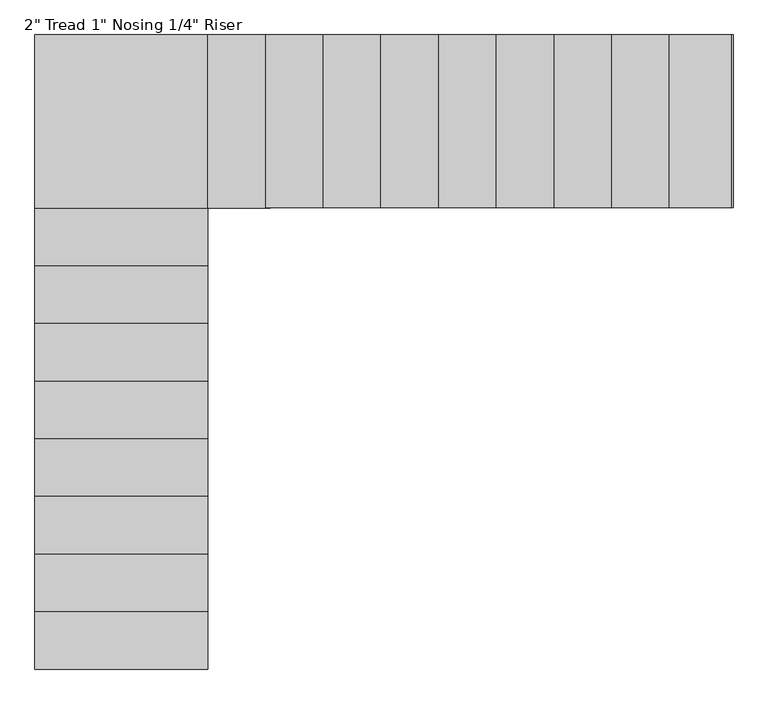
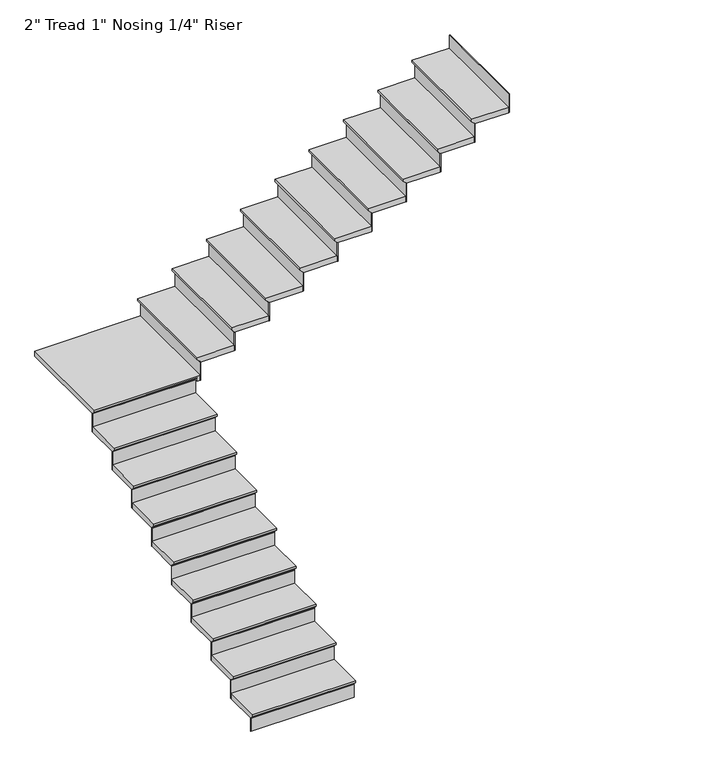
"""IFC4 building model written with IfcOpenShell, lengths in millimetres: stair flight geometry."""

from ifc_helpers import new_model, si_unit, origin, place, context, project, spatial, faceted_brep, source, transform, mapped, element, save


def stair_flight_ebba5fc4(model_context):
    return source(origin(), model_context, "Body", "Brep", [
        faceted_brep([(-6027.2757327, 1771.427543, 3506.47), (-6027.2757327, 1771.427543, 3525.52), (-6941.6757327, 1771.427543, 3525.52), (-6941.6757327, 1771.427543, 3506.47), (-6027.2757327, 1796.827543, 3481.07), (-6941.6757327, 1796.827543, 3481.07), (-6027.2757327, 2101.627543, 3525.52), (-6941.6757327, 2101.627543, 3525.52), (-6941.6757327, 1796.827543, 3474.72), (-6941.6757327, 2101.627543, 3474.72), (-6027.2757327, 2101.627543, 3474.72), (-6027.2757327, 1796.827543, 3474.72)], [[[0, 1, 2, 3]], [[4, 0, 3, 5]], [[2, 1, 6, 7]], [[8, 9, 10, 11]], [[2, 7, 9, 8, 5, 3]], [[8, 11, 4, 5]], [[6, 1, 0, 4, 11, 10]], [[7, 6, 10, 9]]]),
        faceted_brep([(-6027.2757327, 1796.827543, 3474.72), (-6027.2757327, 1796.827543, 3352.8), (-6027.2757327, 1803.177543, 3352.8), (-6027.2757327, 1803.177543, 3474.72), (-6941.6757327, 1796.827543, 3474.72), (-6941.6757327, 1803.177543, 3474.72), (-6941.6757327, 1803.177543, 3352.8), (-6941.6757327, 1796.827543, 3352.8)], [[[0, 1, 2, 3]], [[4, 5, 6, 7]], [[1, 0, 4, 7]], [[2, 1, 7, 6]], [[3, 2, 6, 5]], [[0, 3, 5, 4]]]),
        faceted_brep([(-6027.2757327, 2101.627543, 3647.44), (-6027.2757327, 2101.627543, 3474.72), (-6027.2757327, 2107.977543, 3474.72), (-6027.2757327, 2107.977543, 3647.44), (-6941.6757327, 2101.627543, 3647.44), (-6941.6757327, 2107.977543, 3647.44), (-6941.6757327, 2107.977543, 3474.72), (-6941.6757327, 2101.627543, 3474.72)], [[[0, 1, 2, 3]], [[4, 5, 6, 7]], [[1, 0, 4, 7]], [[2, 1, 7, 6]], [[3, 2, 6, 5]], [[0, 3, 5, 4]]]),
        faceted_brep([(-6941.6757327, 2076.227543, 3698.24), (-6027.2757327, 2076.227543, 3698.24), (-6027.2757327, 2406.427543, 3698.24), (-6941.6757327, 2406.427543, 3698.24), (-6941.6757327, 2101.627543, 3647.44), (-6941.6757327, 2406.427543, 3647.44), (-6027.2757327, 2406.427543, 3647.44), (-6027.2757327, 2101.627543, 3647.44), (-6941.6757327, 2101.627543, 3653.79), (-6941.6757327, 2076.227543, 3679.19), (-6027.2757327, 2101.627543, 3653.79), (-6027.2757327, 2076.227543, 3679.19)], [[[0, 1, 2, 3]], [[4, 5, 6, 7]], [[0, 3, 5, 4, 8, 9]], [[4, 7, 10, 8]], [[2, 1, 11, 10, 7, 6]], [[3, 2, 6, 5]], [[11, 1, 0, 9]], [[10, 11, 9, 8]]]),
        faceted_brep([(-6027.2757327, 2406.427543, 3820.16), (-6027.2757327, 2406.427543, 3647.44), (-6027.2757327, 2412.777543, 3647.44), (-6027.2757327, 2412.777543, 3820.16), (-6941.6757327, 2406.427543, 3820.16), (-6941.6757327, 2412.777543, 3820.16), (-6941.6757327, 2412.777543, 3647.44), (-6941.6757327, 2406.427543, 3647.44)], [[[0, 1, 2, 3]], [[4, 5, 6, 7]], [[1, 0, 4, 7]], [[2, 1, 7, 6]], [[3, 2, 6, 5]], [[0, 3, 5, 4]]]),
        faceted_brep([(-6941.6757327, 2381.027543, 3870.96), (-6027.2757327, 2381.027543, 3870.96), (-6027.2757327, 2711.227543, 3870.96), (-6941.6757327, 2711.227543, 3870.96), (-6941.6757327, 2406.427543, 3820.16), (-6941.6757327, 2711.227543, 3820.16), (-6027.2757327, 2711.227543, 3820.16), (-6027.2757327, 2406.427543, 3820.16), (-6941.6757327, 2406.427543, 3826.51), (-6941.6757327, 2381.027543, 3851.91), (-6027.2757327, 2406.427543, 3826.51), (-6027.2757327, 2381.027543, 3851.91)], [[[0, 1, 2, 3]], [[4, 5, 6, 7]], [[0, 3, 5, 4, 8, 9]], [[4, 7, 10, 8]], [[2, 1, 11, 10, 7, 6]], [[3, 2, 6, 5]], [[11, 1, 0, 9]], [[10, 11, 9, 8]]]),
        faceted_brep([(-6027.2757327, 2711.227543, 3992.88), (-6027.2757327, 2711.227543, 3820.16), (-6027.2757327, 2717.577543, 3820.16), (-6027.2757327, 2717.577543, 3992.88), (-6941.6757327, 2711.227543, 3992.88), (-6941.6757327, 2717.577543, 3992.88), (-6941.6757327, 2717.577543, 3820.16), (-6941.6757327, 2711.227543, 3820.16)], [[[0, 1, 2, 3]], [[4, 5, 6, 7]], [[1, 0, 4, 7]], [[2, 1, 7, 6]], [[3, 2, 6, 5]], [[0, 3, 5, 4]]]),
        faceted_brep([(-6941.6757327, 2685.827543, 4043.68), (-6027.2757327, 2685.827543, 4043.68), (-6027.2757327, 3016.027543, 4043.68), (-6941.6757327, 3016.027543, 4043.68), (-6941.6757327, 2711.227543, 3992.88), (-6941.6757327, 3016.027543, 3992.88), (-6027.2757327, 3016.027543, 3992.88), (-6027.2757327, 2711.227543, 3992.88), (-6941.6757327, 2711.227543, 3999.23), (-6941.6757327, 2685.827543, 4024.63), (-6027.2757327, 2711.227543, 3999.23), (-6027.2757327, 2685.827543, 4024.63)], [[[0, 1, 2, 3]], [[4, 5, 6, 7]], [[0, 3, 5, 4, 8, 9]], [[4, 7, 10, 8]], [[2, 1, 11, 10, 7, 6]], [[3, 2, 6, 5]], [[11, 1, 0, 9]], [[10, 11, 9, 8]]]),
        faceted_brep([(-6027.2757327, 3016.027543, 4165.6), (-6027.2757327, 3016.027543, 3992.88), (-6027.2757327, 3022.377543, 3992.88), (-6027.2757327, 3022.377543, 4165.6), (-6941.6757327, 3016.027543, 4165.6), (-6941.6757327, 3022.377543, 4165.6), (-6941.6757327, 3022.377543, 3992.88), (-6941.6757327, 3016.027543, 3992.88)], [[[0, 1, 2, 3]], [[4, 5, 6, 7]], [[1, 0, 4, 7]], [[2, 1, 7, 6]], [[3, 2, 6, 5]], [[0, 3, 5, 4]]]),
        faceted_brep([(-6941.6757327, 2990.627543, 4216.4), (-6027.2757327, 2990.627543, 4216.4), (-6027.2757327, 3320.827543, 4216.4), (-6941.6757327, 3320.827543, 4216.4), (-6941.6757327, 3016.027543, 4165.6), (-6941.6757327, 3320.827543, 4165.6), (-6027.2757327, 3320.827543, 4165.6), (-6027.2757327, 3016.027543, 4165.6), (-6941.6757327, 3016.027543, 4171.95), (-6941.6757327, 2990.627543, 4197.35), (-6027.2757327, 3016.027543, 4171.95), (-6027.2757327, 2990.627543, 4197.35)], [[[0, 1, 2, 3]], [[4, 5, 6, 7]], [[0, 3, 5, 4, 8, 9]], [[4, 7, 10, 8]], [[2, 1, 11, 10, 7, 6]], [[3, 2, 6, 5]], [[11, 1, 0, 9]], [[10, 11, 9, 8]]]),
        faceted_brep([(-6027.2757327, 3320.827543, 4338.32), (-6027.2757327, 3320.827543, 4165.6), (-6027.2757327, 3327.177543, 4165.6), (-6027.2757327, 3327.177543, 4338.32), (-6941.6757327, 3320.827543, 4338.32), (-6941.6757327, 3327.177543, 4338.32), (-6941.6757327, 3327.177543, 4165.6), (-6941.6757327, 3320.827543, 4165.6)], [[[0, 1, 2, 3]], [[4, 5, 6, 7]], [[1, 0, 4, 7]], [[2, 1, 7, 6]], [[3, 2, 6, 5]], [[0, 3, 5, 4]]]),
        faceted_brep([(-6941.6757327, 3295.427543, 4389.12), (-6027.2757327, 3295.427543, 4389.12), (-6027.2757327, 3625.627543, 4389.12), (-6941.6757327, 3625.627543, 4389.12), (-6941.6757327, 3320.827543, 4338.32), (-6941.6757327, 3625.627543, 4338.32), (-6027.2757327, 3625.627543, 4338.32), (-6027.2757327, 3320.827543, 4338.32), (-6941.6757327, 3320.827543, 4344.67), (-6941.6757327, 3295.427543, 4370.07), (-6027.2757327, 3320.827543, 4344.67), (-6027.2757327, 3295.427543, 4370.07)], [[[0, 1, 2, 3]], [[4, 5, 6, 7]], [[0, 3, 5, 4, 8, 9]], [[4, 7, 10, 8]], [[2, 1, 11, 10, 7, 6]], [[3, 2, 6, 5]], [[11, 1, 0, 9]], [[10, 11, 9, 8]]]),
        faceted_brep([(-6027.2757327, 3625.627543, 4511.04), (-6027.2757327, 3625.627543, 4338.32), (-6027.2757327, 3631.977543, 4338.32), (-6027.2757327, 3631.977543, 4511.04), (-6941.6757327, 3625.627543, 4511.04), (-6941.6757327, 3631.977543, 4511.04), (-6941.6757327, 3631.977543, 4338.32), (-6941.6757327, 3625.627543, 4338.32)], [[[0, 1, 2, 3]], [[4, 5, 6, 7]], [[1, 0, 4, 7]], [[2, 1, 7, 6]], [[3, 2, 6, 5]], [[0, 3, 5, 4]]]),
        faceted_brep([(-6941.6757327, 3600.227543, 4561.84), (-6027.2757327, 3600.227543, 4561.84), (-6027.2757327, 3930.427543, 4561.84), (-6941.6757327, 3930.427543, 4561.84), (-6941.6757327, 3625.627543, 4511.04), (-6941.6757327, 3930.427543, 4511.04), (-6027.2757327, 3930.427543, 4511.04), (-6027.2757327, 3625.627543, 4511.04), (-6941.6757327, 3625.627543, 4517.39), (-6941.6757327, 3600.227543, 4542.79), (-6027.2757327, 3625.627543, 4517.39), (-6027.2757327, 3600.227543, 4542.79)], [[[0, 1, 2, 3]], [[4, 5, 6, 7]], [[0, 3, 5, 4, 8, 9]], [[4, 7, 10, 8]], [[2, 1, 11, 10, 7, 6]], [[3, 2, 6, 5]], [[11, 1, 0, 9]], [[10, 11, 9, 8]]]),
        faceted_brep([(-6027.2757327, 3930.427543, 4683.76), (-6027.2757327, 3930.427543, 4511.04), (-6027.2757327, 3936.777543, 4511.04), (-6027.2757327, 3936.777543, 4683.76), (-6941.6757327, 3930.427543, 4683.76), (-6941.6757327, 3936.777543, 4683.76), (-6941.6757327, 3936.777543, 4511.04), (-6941.6757327, 3930.427543, 4511.04)], [[[0, 1, 2, 3]], [[4, 5, 6, 7]], [[1, 0, 4, 7]], [[2, 1, 7, 6]], [[3, 2, 6, 5]], [[0, 3, 5, 4]]]),
        faceted_brep([(-6941.6757327, 3905.027543, 4734.56), (-6027.2757327, 3905.027543, 4734.56), (-6027.2757327, 4235.227543, 4734.56), (-6941.6757327, 4235.227543, 4734.56), (-6941.6757327, 3930.427543, 4683.76), (-6941.6757327, 4235.227543, 4683.76), (-6027.2757327, 4235.227543, 4683.76), (-6027.2757327, 3930.427543, 4683.76), (-6941.6757327, 3930.427543, 4690.11), (-6941.6757327, 3905.027543, 4715.51), (-6027.2757327, 3930.427543, 4690.11), (-6027.2757327, 3905.027543, 4715.51)], [[[0, 1, 2, 3]], [[4, 5, 6, 7]], [[0, 3, 5, 4, 8, 9]], [[4, 7, 10, 8]], [[2, 1, 11, 10, 7, 6]], [[3, 2, 6, 5]], [[11, 1, 0, 9]], [[10, 11, 9, 8]]]),
        faceted_brep([(-6027.2757327, 4235.227543, 4856.48), (-6027.2757327, 4235.227543, 4683.76), (-6027.2757327, 4241.577543, 4683.76), (-6027.2757327, 4241.577543, 4856.48), (-6941.6757327, 4235.227543, 4856.48), (-6941.6757327, 4241.577543, 4856.48), (-6941.6757327, 4241.577543, 4683.76), (-6941.6757327, 4235.227543, 4683.76)], [[[0, 1, 2, 3]], [[4, 5, 6, 7]], [[1, 0, 4, 7]], [[2, 1, 7, 6]], [[3, 2, 6, 5]], [[0, 3, 5, 4]]]),
        faceted_brep([(-6001.8757327, 5124.227543, 4907.28), (-6941.6757327, 5124.227543, 4907.28), (-6941.6757327, 4209.827543, 4907.28), (-6001.8757327, 4209.827543, 4907.28), (-6941.6757327, 5124.227543, 4856.48), (-6001.8757327, 5124.227543, 4856.48), (-6001.8757327, 4209.827543, 4856.48), (-6027.2757327, 4209.827543, 4856.48), (-6027.2757327, 4235.227543, 4856.48), (-6941.6757327, 4235.227543, 4856.48), (-6941.6757327, 4235.227543, 4862.83), (-6941.6757327, 4209.827543, 4888.23), (-6027.2757327, 4235.227543, 4862.83), (-6027.2757327, 4209.827543, 4888.23)], [[[0, 1, 2, 3]], [[4, 5, 6, 7, 8, 9]], [[1, 0, 5, 4]], [[2, 1, 4, 9, 10, 11]], [[9, 8, 12, 10]], [[8, 7, 13, 12]], [[3, 2, 11, 13, 7, 6]], [[0, 3, 6, 5]], [[11, 10, 12, 13]]]),
        faceted_brep([(-6001.8757327, 4209.827543, 5029.2), (-6001.8757327, 4209.827543, 4856.48), (-5995.5257327, 4209.827543, 4856.48), (-5995.5257327, 4209.827543, 5029.2), (-6001.8757327, 5124.227543, 5029.2), (-5995.5257327, 5124.227543, 5029.2), (-5995.5257327, 5124.227543, 4856.48), (-6001.8757327, 5124.227543, 4856.48)], [[[0, 1, 2, 3]], [[4, 5, 6, 7]], [[1, 0, 4, 7]], [[2, 1, 7, 6]], [[3, 2, 6, 5]], [[0, 3, 5, 4]]]),
        faceted_brep([(-6027.2757327, 5124.227543, 5080.0), (-6027.2757327, 4209.827543, 5080.0), (-5697.0757327, 4209.827543, 5080.0), (-5697.0757327, 5124.227543, 5080.0), (-6001.8757327, 5124.227543, 5029.2), (-5697.0757327, 5124.227543, 5029.2), (-5697.0757327, 4209.827543, 5029.2), (-6001.8757327, 4209.827543, 5029.2), (-6001.8757327, 5124.227543, 5035.55), (-6027.2757327, 5124.227543, 5060.95), (-6001.8757327, 4209.827543, 5035.55), (-6027.2757327, 4209.827543, 5060.95)], [[[0, 1, 2, 3]], [[4, 5, 6, 7]], [[0, 3, 5, 4, 8, 9]], [[4, 7, 10, 8]], [[2, 1, 11, 10, 7, 6]], [[3, 2, 6, 5]], [[11, 1, 0, 9]], [[10, 11, 9, 8]]]),
        faceted_brep([(-5697.0757327, 4209.827543, 5201.92), (-5697.0757327, 4209.827543, 5029.2), (-5690.7257327, 4209.827543, 5029.2), (-5690.7257327, 4209.827543, 5201.92), (-5697.0757327, 5124.227543, 5201.92), (-5690.7257327, 5124.227543, 5201.92), (-5690.7257327, 5124.227543, 5029.2), (-5697.0757327, 5124.227543, 5029.2)], [[[0, 1, 2, 3]], [[4, 5, 6, 7]], [[1, 0, 4, 7]], [[2, 1, 7, 6]], [[3, 2, 6, 5]], [[0, 3, 5, 4]]]),
        faceted_brep([(-5722.4757327, 5124.227543, 5252.72), (-5722.4757327, 4209.827543, 5252.72), (-5392.2757327, 4209.827543, 5252.72), (-5392.2757327, 5124.227543, 5252.72), (-5697.0757327, 5124.227543, 5201.92), (-5392.2757327, 5124.227543, 5201.92), (-5392.2757327, 4209.827543, 5201.92), (-5697.0757327, 4209.827543, 5201.92), (-5697.0757327, 5124.227543, 5208.27), (-5722.4757327, 5124.227543, 5233.67), (-5697.0757327, 4209.827543, 5208.27), (-5722.4757327, 4209.827543, 5233.67)], [[[0, 1, 2, 3]], [[4, 5, 6, 7]], [[0, 3, 5, 4, 8, 9]], [[4, 7, 10, 8]], [[2, 1, 11, 10, 7, 6]], [[3, 2, 6, 5]], [[11, 1, 0, 9]], [[10, 11, 9, 8]]]),
        faceted_brep([(-5392.2757327, 4209.827543, 5374.64), (-5392.2757327, 4209.827543, 5201.92), (-5385.9257327, 4209.827543, 5201.92), (-5385.9257327, 4209.827543, 5374.64), (-5392.2757327, 5124.227543, 5374.64), (-5385.9257327, 5124.227543, 5374.64), (-5385.9257327, 5124.227543, 5201.92), (-5392.2757327, 5124.227543, 5201.92)], [[[0, 1, 2, 3]], [[4, 5, 6, 7]], [[1, 0, 4, 7]], [[2, 1, 7, 6]], [[3, 2, 6, 5]], [[0, 3, 5, 4]]]),
        faceted_brep([(-5417.6757327, 5124.227543, 5425.44), (-5417.6757327, 4209.827543, 5425.44), (-5087.4757327, 4209.827543, 5425.44), (-5087.4757327, 5124.227543, 5425.44), (-5392.2757327, 5124.227543, 5374.64), (-5087.4757327, 5124.227543, 5374.64), (-5087.4757327, 4209.827543, 5374.64), (-5392.2757327, 4209.827543, 5374.64), (-5392.2757327, 5124.227543, 5380.99), (-5417.6757327, 5124.227543, 5406.39), (-5392.2757327, 4209.827543, 5380.99), (-5417.6757327, 4209.827543, 5406.39)], [[[0, 1, 2, 3]], [[4, 5, 6, 7]], [[0, 3, 5, 4, 8, 9]], [[4, 7, 10, 8]], [[2, 1, 11, 10, 7, 6]], [[3, 2, 6, 5]], [[11, 1, 0, 9]], [[10, 11, 9, 8]]]),
        faceted_brep([(-5087.4757327, 4209.827543, 5547.36), (-5087.4757327, 4209.827543, 5374.64), (-5081.1257327, 4209.827543, 5374.64), (-5081.1257327, 4209.827543, 5547.36), (-5087.4757327, 5124.227543, 5547.36), (-5081.1257327, 5124.227543, 5547.36), (-5081.1257327, 5124.227543, 5374.64), (-5087.4757327, 5124.227543, 5374.64)], [[[0, 1, 2, 3]], [[4, 5, 6, 7]], [[1, 0, 4, 7]], [[2, 1, 7, 6]], [[3, 2, 6, 5]], [[0, 3, 5, 4]]]),
        faceted_brep([(-5112.8757327, 5124.227543, 5598.16), (-5112.8757327, 4209.827543, 5598.16), (-4782.6757327, 4209.827543, 5598.16), (-4782.6757327, 5124.227543, 5598.16), (-5087.4757327, 5124.227543, 5547.36), (-4782.6757327, 5124.227543, 5547.36), (-4782.6757327, 4209.827543, 5547.36), (-5087.4757327, 4209.827543, 5547.36), (-5087.4757327, 5124.227543, 5553.71), (-5112.8757327, 5124.227543, 5579.11), (-5087.4757327, 4209.827543, 5553.71), (-5112.8757327, 4209.827543, 5579.11)], [[[0, 1, 2, 3]], [[4, 5, 6, 7]], [[0, 3, 5, 4, 8, 9]], [[4, 7, 10, 8]], [[2, 1, 11, 10, 7, 6]], [[3, 2, 6, 5]], [[11, 1, 0, 9]], [[10, 11, 9, 8]]]),
        faceted_brep([(-4782.6757327, 4209.827543, 5720.08), (-4782.6757327, 4209.827543, 5547.36), (-4776.3257327, 4209.827543, 5547.36), (-4776.3257327, 4209.827543, 5720.08), (-4782.6757327, 5124.227543, 5720.08), (-4776.3257327, 5124.227543, 5720.08), (-4776.3257327, 5124.227543, 5547.36), (-4782.6757327, 5124.227543, 5547.36)], [[[0, 1, 2, 3]], [[4, 5, 6, 7]], [[1, 0, 4, 7]], [[2, 1, 7, 6]], [[3, 2, 6, 5]], [[0, 3, 5, 4]]]),
        faceted_brep([(-4808.0757327, 5124.227543, 5770.88), (-4808.0757327, 4209.827543, 5770.88), (-4477.8757327, 4209.827543, 5770.88), (-4477.8757327, 5124.227543, 5770.88), (-4782.6757327, 5124.227543, 5720.08), (-4477.8757327, 5124.227543, 5720.08), (-4477.8757327, 4209.827543, 5720.08), (-4782.6757327, 4209.827543, 5720.08), (-4782.6757327, 5124.227543, 5726.43), (-4808.0757327, 5124.227543, 5751.83), (-4782.6757327, 4209.827543, 5726.43), (-4808.0757327, 4209.827543, 5751.83)], [[[0, 1, 2, 3]], [[4, 5, 6, 7]], [[0, 3, 5, 4, 8, 9]], [[4, 7, 10, 8]], [[2, 1, 11, 10, 7, 6]], [[3, 2, 6, 5]], [[11, 1, 0, 9]], [[10, 11, 9, 8]]]),
        faceted_brep([(-4477.8757327, 4209.827543, 5892.8), (-4477.8757327, 4209.827543, 5720.08), (-4471.5257327, 4209.827543, 5720.08), (-4471.5257327, 4209.827543, 5892.8), (-4477.8757327, 5124.227543, 5892.8), (-4471.5257327, 5124.227543, 5892.8), (-4471.5257327, 5124.227543, 5720.08), (-4477.8757327, 5124.227543, 5720.08)], [[[0, 1, 2, 3]], [[4, 5, 6, 7]], [[1, 0, 4, 7]], [[2, 1, 7, 6]], [[3, 2, 6, 5]], [[0, 3, 5, 4]]]),
        faceted_brep([(-4503.2757327, 5124.227543, 5943.6), (-4503.2757327, 4209.827543, 5943.6), (-4173.0757327, 4209.827543, 5943.6), (-4173.0757327, 5124.227543, 5943.6), (-4477.8757327, 5124.227543, 5892.8), (-4173.0757327, 5124.227543, 5892.8), (-4173.0757327, 4209.827543, 5892.8), (-4477.8757327, 4209.827543, 5892.8), (-4477.8757327, 5124.227543, 5899.15), (-4503.2757327, 5124.227543, 5924.55), (-4477.8757327, 4209.827543, 5899.15), (-4503.2757327, 4209.827543, 5924.55)], [[[0, 1, 2, 3]], [[4, 5, 6, 7]], [[0, 3, 5, 4, 8, 9]], [[4, 7, 10, 8]], [[2, 1, 11, 10, 7, 6]], [[3, 2, 6, 5]], [[11, 1, 0, 9]], [[10, 11, 9, 8]]]),
        faceted_brep([(-4173.0757327, 4209.827543, 6065.52), (-4173.0757327, 4209.827543, 5892.8), (-4166.7257327, 4209.827543, 5892.8), (-4166.7257327, 4209.827543, 6065.52), (-4173.0757327, 5124.227543, 6065.52), (-4166.7257327, 5124.227543, 6065.52), (-4166.7257327, 5124.227543, 5892.8), (-4173.0757327, 5124.227543, 5892.8)], [[[0, 1, 2, 3]], [[4, 5, 6, 7]], [[1, 0, 4, 7]], [[2, 1, 7, 6]], [[3, 2, 6, 5]], [[0, 3, 5, 4]]]),
        faceted_brep([(-4198.4757327, 5124.227543, 6116.32), (-4198.4757327, 4209.827543, 6116.32), (-3868.2757327, 4209.827543, 6116.32), (-3868.2757327, 5124.227543, 6116.32), (-4173.0757327, 5124.227543, 6065.52), (-3868.2757327, 5124.227543, 6065.52), (-3868.2757327, 4209.827543, 6065.52), (-4173.0757327, 4209.827543, 6065.52), (-4173.0757327, 5124.227543, 6071.87), (-4198.4757327, 5124.227543, 6097.27), (-4173.0757327, 4209.827543, 6071.87), (-4198.4757327, 4209.827543, 6097.27)], [[[0, 1, 2, 3]], [[4, 5, 6, 7]], [[0, 3, 5, 4, 8, 9]], [[4, 7, 10, 8]], [[2, 1, 11, 10, 7, 6]], [[3, 2, 6, 5]], [[11, 1, 0, 9]], [[10, 11, 9, 8]]]),
        faceted_brep([(-3868.2757327, 4209.827543, 6238.24), (-3868.2757327, 4209.827543, 6065.52), (-3861.9257327, 4209.827543, 6065.52), (-3861.9257327, 4209.827543, 6238.24), (-3868.2757327, 5124.227543, 6238.24), (-3861.9257327, 5124.227543, 6238.24), (-3861.9257327, 5124.227543, 6065.52), (-3868.2757327, 5124.227543, 6065.52)], [[[0, 1, 2, 3]], [[4, 5, 6, 7]], [[1, 0, 4, 7]], [[2, 1, 7, 6]], [[3, 2, 6, 5]], [[0, 3, 5, 4]]]),
        faceted_brep([(-3893.6757327, 5124.227543, 6289.04), (-3893.6757327, 4209.827543, 6289.04), (-3563.4757327, 4209.827543, 6289.04), (-3563.4757327, 5124.227543, 6289.04), (-3868.2757327, 5124.227543, 6238.24), (-3563.4757327, 5124.227543, 6238.24), (-3563.4757327, 4209.827543, 6238.24), (-3868.2757327, 4209.827543, 6238.24), (-3868.2757327, 5124.227543, 6244.59), (-3893.6757327, 5124.227543, 6269.99), (-3868.2757327, 4209.827543, 6244.59), (-3893.6757327, 4209.827543, 6269.99)], [[[0, 1, 2, 3]], [[4, 5, 6, 7]], [[0, 3, 5, 4, 8, 9]], [[4, 7, 10, 8]], [[2, 1, 11, 10, 7, 6]], [[3, 2, 6, 5]], [[11, 1, 0, 9]], [[10, 11, 9, 8]]]),
        faceted_brep([(-3563.4757327, 4209.827543, 6410.96), (-3563.4757327, 4209.827543, 6238.24), (-3557.1257327, 4209.827543, 6238.24), (-3557.1257327, 4209.827543, 6410.96), (-3563.4757327, 5124.227543, 6410.96), (-3557.1257327, 5124.227543, 6410.96), (-3557.1257327, 5124.227543, 6238.24), (-3563.4757327, 5124.227543, 6238.24)], [[[0, 1, 2, 3]], [[4, 5, 6, 7]], [[1, 0, 4, 7]], [[2, 1, 7, 6]], [[3, 2, 6, 5]], [[0, 3, 5, 4]]]),
        faceted_brep([(-3258.6757327, 4209.827543, 6583.68), (-3258.6757327, 4209.827543, 6410.96), (-3252.3257327, 4209.827543, 6410.96), (-3252.3257327, 4209.827543, 6583.68), (-3258.6757327, 5124.227543, 6583.68), (-3252.3257327, 5124.227543, 6583.68), (-3252.3257327, 5124.227543, 6410.96), (-3258.6757327, 5124.227543, 6410.96)], [[[0, 1, 2, 3]], [[4, 5, 6, 7]], [[1, 0, 4, 7]], [[2, 1, 7, 6]], [[3, 2, 6, 5]], [[0, 3, 5, 4]]]),
        faceted_brep([(-3588.8757327, 5124.227543, 6461.76), (-3588.8757327, 4209.827543, 6461.76), (-3258.6757327, 4209.827543, 6461.76), (-3258.6757327, 5124.227543, 6461.76), (-3563.4757327, 5124.227543, 6410.96), (-3258.6757327, 5124.227543, 6410.96), (-3258.6757327, 4209.827543, 6410.96), (-3563.4757327, 4209.827543, 6410.96), (-3563.4757327, 5124.227543, 6417.31), (-3588.8757327, 5124.227543, 6442.71), (-3563.4757327, 4209.827543, 6417.31), (-3588.8757327, 4209.827543, 6442.71)], [[[0, 1, 2, 3]], [[4, 5, 6, 7]], [[0, 3, 5, 4, 8, 9]], [[4, 7, 10, 8]], [[2, 1, 11, 10, 7, 6]], [[3, 2, 6, 5]], [[11, 1, 0, 9]], [[10, 11, 9, 8]]]),
    ])


if __name__ == "__main__":
    model = new_model("IFC4")
    model_context = context("Model", 3, world=origin())
    ifc_project = project(units=[si_unit("LENGTHUNIT", "METRE", prefix="MILLI")], contexts=[model_context])
    site = spatial("IfcSite", under=ifc_project)
    building = spatial("IfcBuilding", under=site)
    placement = place(None, origin())
    stair_flight_shape = stair_flight_ebba5fc4(model_context)
    element("IfcStairFlight", 1, ObjectType="2\" Tread 1\" Nosing 1/4\" Riser", at=placement, inside=building, context=model_context, shape_type="MappedRepresentation", body=[
        mapped(stair_flight_shape, transform((0.0, 0.0, 0.0), x_axis=(1.0, 0.0, 0.0), y_axis=(0.0, 1.0, 0.0), z_axis=(0.0, 0.0, 1.0))),
    ])
    save(model, "model.ifc")

# Revit data of these elements
# Element 1 (IfcStairFlight, "2\" Tread 1\" Nosing 1/4\" Riser")
#   Materials on its faces: "MARBLE FLOORING"
# Materials
#   "MARBLE FLOORING": class "Generic", colour RGB 120 120 120, transparency 0, Cost = 0
